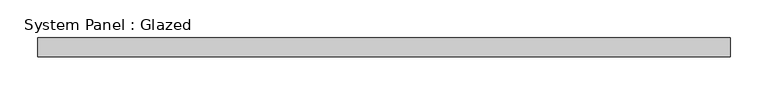
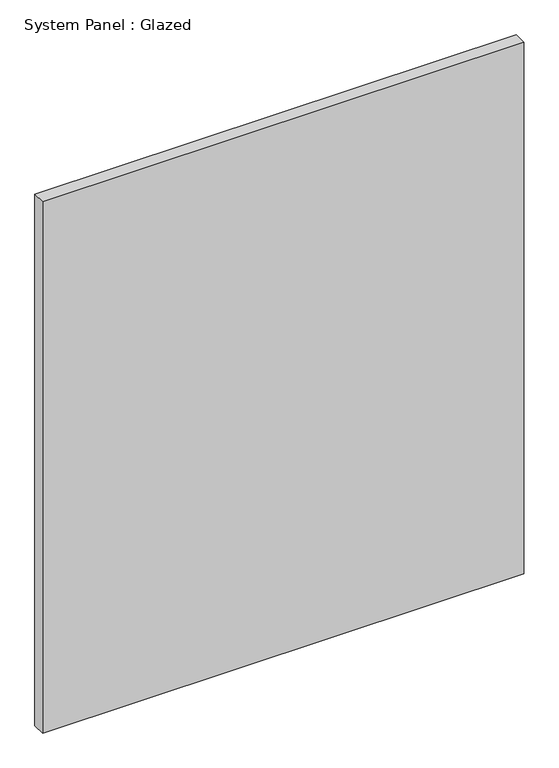
"""IFC4 building model written with IfcOpenShell, lengths in millimetres: plate geometry, System Panel : Glazed."""

from ifc_helpers import new_model, si_unit, origin, origin_with_axes, place, context, project, spatial, polyline, outline, extrude, source, transform, mapped, element, save


def system_panel_glazed_c442566e(model_context):
    return source(origin(), model_context, "Body", "SweptSolid", [
        extrude(outline(polyline([(457.2, 24.5), (-457.2, 24.5), (-457.2, 49.5), (457.2, 49.5), (457.2, 24.5)])), origin_with_axes(), (0.0, 0.0, 1.0), 1066.8),
    ])


if __name__ == "__main__":
    model = new_model("IFC4")
    model_context = context("Model", 3, world=origin())
    ifc_project = project(units=[si_unit("LENGTHUNIT", "METRE", prefix="MILLI")], contexts=[model_context])
    site = spatial("IfcSite", under=ifc_project)
    building = spatial("IfcBuilding", under=site)
    placement = place(None, origin())
    system_panel_glazed_shape = system_panel_glazed_c442566e(model_context)
    element("IfcPlate", 1, ObjectType="System Panel : Glazed", at=placement, inside=building, context=model_context, shape_type="MappedRepresentation", body=[
        mapped(system_panel_glazed_shape, transform((0.0, 0.0, 0.0), x_axis=(1.0, 0.0, 0.0), y_axis=(0.0, 1.0, 0.0), z_axis=(0.0, 0.0, 1.0))),
    ])
    save(model, "model.ifc")

# Revit data of these elements
# Type "System Panel : Glazed"
#   Construction Type Id = "GSP4R"
#   Analytic Construction = "1/8 in Pilkington single glazing"
#   Visual Light Transmittance = 0.9
#   Solar Heat Gain Coefficient = 0.86
#   Heat Transfer Coefficient (U) = 6.7069 W/(m²·K)
#   Define Thermal Properties by = 1
# Element 1 (IfcPlate, "System Panel : Glazed")
#   Materials on its faces: "Glass"
# Materials
#   "Glass": class "Glass", colour RGB 0 128 192, transparency 0.9, Description = "Soda Lime Glass", Cost = 0
